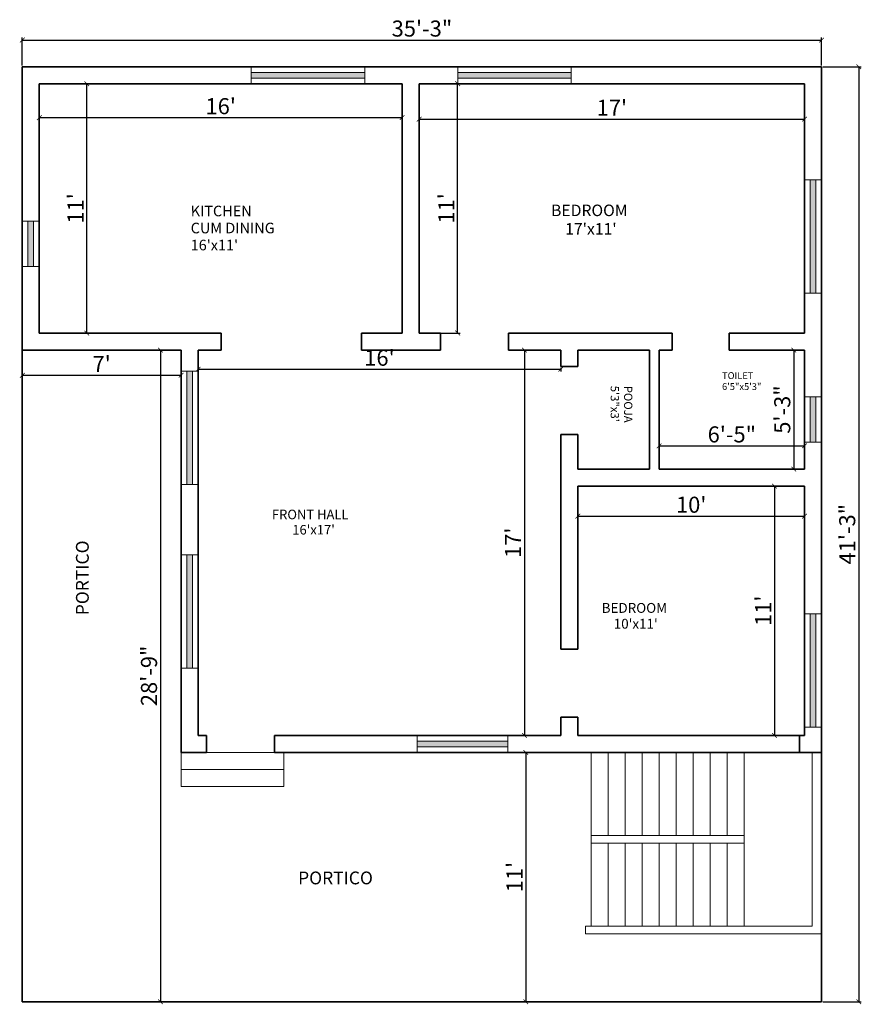
# Model space of a CAD drawing. Units: inches. Extents: x 3799 to 20199, y 1682 to 8087.
# Tile 14 of 30: x 7648 to 8094, y 5909 to 6430. Entities that reach past the tile are written whole.
import ezdxf

# ---------------------------------------------------------------- set-up
doc = ezdxf.new("R2010")
doc.units = ezdxf.units.IN
for name, color, linetype, lineweight in [('A-ANNO-DIMS', 2, 'Continuous', 18), ('A-AREA-IDEN', 7, 'Continuous', 18), ('A-FLOR-STRS', 41, 'Continuous', 18), ('A-GLAZ', 152, 'Continuous', 18), ('A-WALL', 7, 'Continuous', 35), ('A-WALL-PATT', 252, 'Continuous', 13)]:
    doc.layers.add(name, color=color, linetype=linetype, lineweight=lineweight)
doc.styles.get("Standard").update_dxf_attribs({"font": 'arial.ttf'})
doc.dimstyles.new('ISO-25', dxfattribs={"dimtxt": 8.5, "dimasz": 2.5, "dimexe": 1.25, "dimexo": 0.625, "dimtad": 1, "dimdec": 0, "dimlunit": 3, "dimtxsty": 'Standard', "dimblk": 'ARCHTICK', "dimcen": 2.5, "dimadec": 0, "dimazin": 0, "dimtfac": 1, "dimtdec": 0, "dimtmove": 0, "dimatfit": 3, "dimfxl": 1, "dimarcsym": 0})

# ---------------------------------------------------------------- blocks, each defined once
blk = doc.blocks.new('_ArchTick')
at = {"color": 0, "linetype": 'ByBlock', "const_width": 0.15}
blk.add_lwpolyline([(-0.5, -0.5), (0.5, 0.5)], dxfattribs=at)
blk = doc.blocks.new('*D200')
at = {"layer": 'A-ANNO-DIMS', "color": 0, "lineweight": -2, "transparency": 16777216}
for p, q in [((7658.6, 6395.56), (7658.6, 6376.97)), ((7850.6, 6395.56), (7850.6, 6376.97)), ((7658.6, 6378.22), (7850.6, 6378.22))]:
    blk.add_line(p, q, dxfattribs=at)
at = {"layer": 'Defpoints', "color": 0, "transparency": 16777216}
for p in [(7658.6, 6396.18), (7850.6, 6396.18), (7850.6, 6378.22)]:
    blk.add_point(p, dxfattribs=at)
at = {"layer": 'A-ANNO-DIMS', "color": 0, "lineweight": -2, "transparency": 16777216, "xscale": 2.5, "yscale": 2.5, "zscale": 2.5, "rotation": 180}
blk.add_blockref('_ArchTick', (7658.6, 6378.22), dxfattribs=at)
at = {"layer": 'A-ANNO-DIMS', "color": 0, "lineweight": -2, "transparency": 16777216, "xscale": 2.5, "yscale": 2.5, "zscale": 2.5}
blk.add_blockref('_ArchTick', (7850.6, 6378.22), dxfattribs=at)
at = {"layer": 'A-ANNO-DIMS', "color": 0, "transparency": 16777216, "insert": (7754.6, 6383.19), "char_height": 8.5, "attachment_point": 5}
blk.add_mtext("16'", dxfattribs=at)
blk = doc.blocks.new('*D201')
at = {"layer": 'A-ANNO-DIMS', "color": 0, "lineweight": -2, "transparency": 16777216}
for p, q in [((7659.22, 6396.18), (7685, 6396.18)), ((7683.75, 6264.18), (7683.75, 6396.18)), ((7659.22, 6264.18), (7685, 6264.18))]:
    blk.add_line(p, q, dxfattribs=at)
at = {"layer": 'Defpoints', "color": 0, "transparency": 16777216}
for p in [(7658.6, 6396.18), (7683.75, 6396.18), (7658.6, 6264.18)]:
    blk.add_point(p, dxfattribs=at)
at = {"layer": 'A-ANNO-DIMS', "color": 0, "lineweight": -2, "transparency": 16777216, "xscale": 2.5, "yscale": 2.5, "zscale": 2.5}
for p, rotation in [((7683.75, 6396.18), 90), ((7683.75, 6264.18), 270)]:
    blk.add_blockref('_ArchTick', p, dxfattribs=dict(at, rotation=rotation))
at = {"layer": 'A-ANNO-DIMS', "color": 0, "transparency": 16777216, "insert": (7678.86, 6330.18), "char_height": 8.5, "attachment_point": 5, "rotation": 90}
blk.add_mtext("11'", dxfattribs=at)
blk = doc.blocks.new('*D202')
at = {"layer": 'A-ANNO-DIMS', "color": 0, "lineweight": -2, "transparency": 16777216}
for p, q in [((7860.22, 6396.18), (7881.25, 6396.18)), ((7880, 6264.18), (7880, 6396.18)), ((7860.22, 6264.18), (7881.25, 6264.18))]:
    blk.add_line(p, q, dxfattribs=at)
at = {"layer": 'Defpoints', "color": 0, "transparency": 16777216}
for p in [(7859.6, 6396.18), (7880, 6396.18), (7859.6, 6264.18)]:
    blk.add_point(p, dxfattribs=at)
at = {"layer": 'A-ANNO-DIMS', "color": 0, "lineweight": -2, "transparency": 16777216, "xscale": 2.5, "yscale": 2.5, "zscale": 2.5}
for p, rotation in [((7880, 6396.18), 90), ((7880, 6264.18), 270)]:
    blk.add_blockref('_ArchTick', p, dxfattribs=dict(at, rotation=rotation))
at = {"layer": 'A-ANNO-DIMS', "color": 0, "transparency": 16777216, "insert": (7875.11, 6330.18), "char_height": 8.5, "attachment_point": 5, "rotation": 90}
blk.add_mtext("11'", dxfattribs=at)
blk = doc.blocks.new('*D203')
at = {"layer": 'A-ANNO-DIMS', "color": 0, "lineweight": -2, "transparency": 16777216}
for p, q in [((7859.6, 6395.56), (7859.6, 6376.2)), ((8063.6, 6395.56), (8063.6, 6376.2)), ((7859.6, 6377.45), (8063.6, 6377.45))]:
    blk.add_line(p, q, dxfattribs=at)
at = {"layer": 'Defpoints', "color": 0, "transparency": 16777216}
for p in [(7859.6, 6396.18), (8063.6, 6396.18), (8063.6, 6377.45)]:
    blk.add_point(p, dxfattribs=at)
at = {"layer": 'A-ANNO-DIMS', "color": 0, "lineweight": -2, "transparency": 16777216, "xscale": 2.5, "yscale": 2.5, "zscale": 2.5, "rotation": 180}
blk.add_blockref('_ArchTick', (7859.6, 6377.45), dxfattribs=at)
at = {"layer": 'A-ANNO-DIMS', "color": 0, "lineweight": -2, "transparency": 16777216, "xscale": 2.5, "yscale": 2.5, "zscale": 2.5}
blk.add_blockref('_ArchTick', (8063.6, 6377.45), dxfattribs=at)
at = {"layer": 'A-ANNO-DIMS', "color": 0, "transparency": 16777216, "insert": (7961.6, 6382.34), "char_height": 8.5, "attachment_point": 5}
blk.add_mtext("17'", dxfattribs=at)
blk = doc.blocks.new('*D204')
at = {"layer": 'A-ANNO-DIMS', "color": 0, "lineweight": -2, "transparency": 16777216}
for p, q in [((7986.6, 6192.81), (7986.6, 6205.71)), ((7986.6, 6204.46), (8063.6, 6204.46)), ((8063.6, 6192.81), (8063.6, 6205.71))]:
    blk.add_line(p, q, dxfattribs=at)
at = {"layer": 'Defpoints', "color": 0, "transparency": 16777216}
for p in [(8063.6, 6204.46), (7986.6, 6192.18), (8063.6, 6192.18)]:
    blk.add_point(p, dxfattribs=at)
at = {"layer": 'A-ANNO-DIMS', "color": 0, "lineweight": -2, "transparency": 16777216, "xscale": 2.5, "yscale": 2.5, "zscale": 2.5, "rotation": 180}
blk.add_blockref('_ArchTick', (7986.6, 6204.46), dxfattribs=at)
at = {"layer": 'A-ANNO-DIMS', "color": 0, "lineweight": -2, "transparency": 16777216, "xscale": 2.5, "yscale": 2.5, "zscale": 2.5}
blk.add_blockref('_ArchTick', (8063.6, 6204.46), dxfattribs=at)
at = {"layer": 'A-ANNO-DIMS', "color": 0, "transparency": 16777216, "insert": (8025.1, 6209.42), "char_height": 8.5, "attachment_point": 5}
blk.add_mtext('6\'-5"', dxfattribs=at)
blk = doc.blocks.new('*D205')
at = {"layer": 'A-ANNO-DIMS', "color": 0, "lineweight": -2, "transparency": 16777216}
for p, q in [((8062.97, 6255.18), (8056.61, 6255.18)), ((8057.86, 6255.18), (8057.86, 6192.18)), ((8062.97, 6192.18), (8056.61, 6192.18))]:
    blk.add_line(p, q, dxfattribs=at)
at = {"layer": 'Defpoints', "color": 0, "transparency": 16777216}
for p in [(8063.6, 6255.18), (8057.86, 6192.18), (8063.6, 6192.18)]:
    blk.add_point(p, dxfattribs=at)
at = {"layer": 'A-ANNO-DIMS', "color": 0, "lineweight": -2, "transparency": 16777216, "xscale": 2.5, "yscale": 2.5, "zscale": 2.5}
for p, rotation in [((8057.86, 6255.18), 90), ((8057.86, 6192.18), 270)]:
    blk.add_blockref('_ArchTick', p, dxfattribs=dict(at, rotation=rotation))
at = {"layer": 'A-ANNO-DIMS', "color": 0, "transparency": 16777216, "insert": (8052.9, 6223.68), "char_height": 8.5, "attachment_point": 5, "rotation": 90}
blk.add_mtext('5\'-3"', dxfattribs=at)
blk = doc.blocks.new('*D206')
at = {"layer": 'A-ANNO-DIMS', "color": 0, "lineweight": -2, "transparency": 16777216}
for p, q in [((7943.6, 6182.56), (7943.6, 6165.96)), ((8063.6, 6182.56), (8063.6, 6165.96)), ((7943.6, 6167.21), (8063.6, 6167.21))]:
    blk.add_line(p, q, dxfattribs=at)
at = {"layer": 'Defpoints', "color": 0, "transparency": 16777216}
for p in [(7943.6, 6183.18), (8063.6, 6183.18), (8063.6, 6167.21)]:
    blk.add_point(p, dxfattribs=at)
at = {"layer": 'A-ANNO-DIMS', "color": 0, "lineweight": -2, "transparency": 16777216, "xscale": 2.5, "yscale": 2.5, "zscale": 2.5, "rotation": 180}
blk.add_blockref('_ArchTick', (7943.6, 6167.21), dxfattribs=at)
at = {"layer": 'A-ANNO-DIMS', "color": 0, "lineweight": -2, "transparency": 16777216, "xscale": 2.5, "yscale": 2.5, "zscale": 2.5}
blk.add_blockref('_ArchTick', (8063.6, 6167.21), dxfattribs=at)
at = {"layer": 'A-ANNO-DIMS', "color": 0, "transparency": 16777216, "insert": (8003.6, 6172.18), "char_height": 8.5, "attachment_point": 5}
blk.add_mtext("10'", dxfattribs=at)
blk = doc.blocks.new('*D207')
at = {"layer": 'A-ANNO-DIMS', "color": 0, "lineweight": -2, "transparency": 16777216}
for p, q in [((8062.97, 6183.18), (8046.43, 6183.18)), ((8047.68, 6183.18), (8047.68, 6051.18)), ((8062.97, 6051.18), (8046.43, 6051.18))]:
    blk.add_line(p, q, dxfattribs=at)
at = {"layer": 'Defpoints', "color": 0, "transparency": 16777216}
for p in [(8063.6, 6183.18), (8047.68, 6051.18), (8063.6, 6051.18)]:
    blk.add_point(p, dxfattribs=at)
at = {"layer": 'A-ANNO-DIMS', "color": 0, "lineweight": -2, "transparency": 16777216, "xscale": 2.5, "yscale": 2.5, "zscale": 2.5}
for p, rotation in [((8047.68, 6183.18), 90), ((8047.68, 6051.18), 270)]:
    blk.add_blockref('_ArchTick', p, dxfattribs=dict(at, rotation=rotation))
at = {"layer": 'A-ANNO-DIMS', "color": 0, "transparency": 16777216, "insert": (8042.78, 6117.18), "char_height": 8.5, "attachment_point": 5, "rotation": 90}
blk.add_mtext("11'", dxfattribs=at)
blk = doc.blocks.new('*D208')
at = {"layer": 'A-ANNO-DIMS', "color": 0, "lineweight": -2, "transparency": 16777216}
for p, q in [((7742.6, 6244.54), (7742.6, 6246.29)), ((7742.6, 6245.04), (7934.6, 6245.04)), ((7934.6, 6245.81), (7934.6, 6243.79))]:
    blk.add_line(p, q, dxfattribs=at)
at = {"layer": 'Defpoints', "color": 0, "transparency": 16777216}
for p in [(7934.6, 6246.44), (7934.6, 6245.04), (7742.6, 6243.91)]:
    blk.add_point(p, dxfattribs=at)
at = {"layer": 'A-ANNO-DIMS', "color": 0, "lineweight": -2, "transparency": 16777216, "xscale": 2.5, "yscale": 2.5, "zscale": 2.5, "rotation": 180}
blk.add_blockref('_ArchTick', (7742.6, 6245.04), dxfattribs=at)
at = {"layer": 'A-ANNO-DIMS', "color": 0, "lineweight": -2, "transparency": 16777216, "xscale": 2.5, "yscale": 2.5, "zscale": 2.5}
blk.add_blockref('_ArchTick', (7934.6, 6245.04), dxfattribs=at)
at = {"layer": 'A-ANNO-DIMS', "color": 0, "transparency": 16777216, "insert": (7838.6, 6250.01), "char_height": 8.5, "attachment_point": 5}
blk.add_mtext("16'", dxfattribs=at)
blk = doc.blocks.new('*D209')
at = {"layer": 'A-ANNO-DIMS', "color": 0, "lineweight": -2, "transparency": 16777216}
for p, q in [((7907.56, 6255.18), (7916.55, 6255.18)), ((7915.3, 6255.18), (7915.3, 6051.18)), ((7907.17, 6051.18), (7916.55, 6051.18))]:
    blk.add_line(p, q, dxfattribs=at)
at = {"layer": 'Defpoints', "color": 0, "transparency": 16777216}
for p in [(7906.93, 6255.18), (7906.55, 6051.18), (7915.3, 6051.18)]:
    blk.add_point(p, dxfattribs=at)
at = {"layer": 'A-ANNO-DIMS', "color": 0, "lineweight": -2, "transparency": 16777216, "xscale": 2.5, "yscale": 2.5, "zscale": 2.5}
for p, rotation in [((7915.3, 6255.18), 90), ((7915.3, 6051.18), 270)]:
    blk.add_blockref('_ArchTick', p, dxfattribs=dict(at, rotation=rotation))
at = {"layer": 'A-ANNO-DIMS', "color": 0, "transparency": 16777216, "insert": (7910.41, 6153.18), "char_height": 8.5, "attachment_point": 5, "rotation": 90}
blk.add_mtext("17'", dxfattribs=at)
blk = doc.blocks.new('*D210')
at = {"layer": 'A-ANNO-DIMS', "color": 0, "lineweight": -2, "transparency": 16777216}
for p, q in [((7732.97, 6255.18), (7721.46, 6255.18)), ((7722.71, 6255.18), (7722.71, 5910.18)), ((7732.97, 5910.18), (7721.46, 5910.18))]:
    blk.add_line(p, q, dxfattribs=at)
at = {"layer": 'Defpoints', "color": 0, "transparency": 16777216}
for p in [(7733.6, 6255.18), (7722.71, 5910.18), (7733.6, 5910.18)]:
    blk.add_point(p, dxfattribs=at)
at = {"layer": 'A-ANNO-DIMS', "color": 0, "lineweight": -2, "transparency": 16777216, "xscale": 2.5, "yscale": 2.5, "zscale": 2.5}
for p, rotation in [((7722.71, 6255.18), 90), ((7722.71, 5910.18), 270)]:
    blk.add_blockref('_ArchTick', p, dxfattribs=dict(at, rotation=rotation))
at = {"layer": 'A-ANNO-DIMS', "color": 0, "transparency": 16777216, "insert": (7717.74, 6082.68), "char_height": 8.5, "attachment_point": 5, "rotation": 90}
blk.add_mtext('28\'-9"', dxfattribs=at)
blk = doc.blocks.new('*D211')
at = {"layer": 'A-ANNO-DIMS', "color": 0, "lineweight": -2, "transparency": 16777216}
for p, q in [((7649.6, 6254.56), (7649.6, 6240.56)), ((7733.6, 6254.56), (7733.6, 6240.56)), ((7649.6, 6241.81), (7733.6, 6241.81))]:
    blk.add_line(p, q, dxfattribs=at)
at = {"layer": 'Defpoints', "color": 0, "transparency": 16777216}
for p in [(7649.6, 6255.18), (7733.6, 6255.18), (7733.6, 6241.81)]:
    blk.add_point(p, dxfattribs=at)
at = {"layer": 'A-ANNO-DIMS', "color": 0, "lineweight": -2, "transparency": 16777216, "xscale": 2.5, "yscale": 2.5, "zscale": 2.5, "rotation": 180}
blk.add_blockref('_ArchTick', (7649.6, 6241.81), dxfattribs=at)
at = {"layer": 'A-ANNO-DIMS', "color": 0, "lineweight": -2, "transparency": 16777216, "xscale": 2.5, "yscale": 2.5, "zscale": 2.5}
blk.add_blockref('_ArchTick', (7733.6, 6241.81), dxfattribs=at)
at = {"layer": 'A-ANNO-DIMS', "color": 0, "transparency": 16777216, "insert": (7691.6, 6246.69), "char_height": 8.5, "attachment_point": 5}
blk.add_mtext("7'", dxfattribs=at)
blk = doc.blocks.new('*D212')
at = {"layer": 'A-ANNO-DIMS', "color": 0, "lineweight": -2, "transparency": 16777216}
for p, q in [((7907.17, 6042.18), (7917.32, 6042.18)), ((7916.07, 6042.18), (7916.07, 5910.18)), ((7907.17, 5910.18), (7917.32, 5910.18))]:
    blk.add_line(p, q, dxfattribs=at)
at = {"layer": 'Defpoints', "color": 0, "transparency": 16777216}
for p in [(7906.55, 6042.18), (7906.55, 5910.18), (7916.07, 5910.18)]:
    blk.add_point(p, dxfattribs=at)
at = {"layer": 'A-ANNO-DIMS', "color": 0, "lineweight": -2, "transparency": 16777216, "xscale": 2.5, "yscale": 2.5, "zscale": 2.5}
for p, rotation in [((7916.07, 6042.18), 90), ((7916.07, 5910.18), 270)]:
    blk.add_blockref('_ArchTick', p, dxfattribs=dict(at, rotation=rotation))
at = {"layer": 'A-ANNO-DIMS', "color": 0, "transparency": 16777216, "insert": (7911.18, 5976.18), "char_height": 8.5, "attachment_point": 5, "rotation": 90}
blk.add_mtext("11'", dxfattribs=at)
blk = doc.blocks.new('*D213')
at = {"layer": 'A-ANNO-DIMS', "color": 0, "lineweight": -2, "transparency": 16777216}
for p, q in [((8073.22, 6405.18), (8093.49, 6405.18)), ((8092.24, 6405.18), (8092.24, 5910.18)), ((8073.22, 5910.18), (8093.49, 5910.18))]:
    blk.add_line(p, q, dxfattribs=at)
at = {"layer": 'Defpoints', "color": 0, "transparency": 16777216}
for p in [(8072.6, 6405.18), (8072.6, 5910.18), (8092.24, 5910.18)]:
    blk.add_point(p, dxfattribs=at)
at = {"layer": 'A-ANNO-DIMS', "color": 0, "lineweight": -2, "transparency": 16777216, "xscale": 2.5, "yscale": 2.5, "zscale": 2.5}
for p, rotation in [((8092.24, 6405.18), 90), ((8092.24, 5910.18), 270)]:
    blk.add_blockref('_ArchTick', p, dxfattribs=dict(at, rotation=rotation))
at = {"layer": 'A-ANNO-DIMS', "color": 0, "transparency": 16777216, "insert": (8087.27, 6157.68), "char_height": 8.5, "attachment_point": 5, "rotation": 90}
blk.add_mtext('41\'-3"', dxfattribs=at)
blk = doc.blocks.new('*D214')
at = {"layer": 'A-ANNO-DIMS', "color": 0, "lineweight": -2, "transparency": 16777216}
for p, q in [((7649.6, 6405.81), (7649.6, 6420.57)), ((7649.6, 6419.32), (8072.6, 6419.32)), ((8072.6, 6405.81), (8072.6, 6420.57))]:
    blk.add_line(p, q, dxfattribs=at)
at = {"layer": 'Defpoints', "color": 0, "transparency": 16777216}
for p in [(8072.6, 6419.32), (7649.6, 6405.18), (8072.6, 6405.18)]:
    blk.add_point(p, dxfattribs=at)
at = {"layer": 'A-ANNO-DIMS', "color": 0, "lineweight": -2, "transparency": 16777216, "xscale": 2.5, "yscale": 2.5, "zscale": 2.5, "rotation": 180}
blk.add_blockref('_ArchTick', (7649.6, 6419.32), dxfattribs=at)
at = {"layer": 'A-ANNO-DIMS', "color": 0, "lineweight": -2, "transparency": 16777216, "xscale": 2.5, "yscale": 2.5, "zscale": 2.5}
blk.add_blockref('_ArchTick', (8072.6, 6419.32), dxfattribs=at)
at = {"layer": 'A-ANNO-DIMS', "color": 0, "transparency": 16777216, "insert": (7861.1, 6424.28), "char_height": 8.5, "attachment_point": 5}
blk.add_mtext('35\'-3"', dxfattribs=at)
blk = doc.blocks.new('WIN-24IN-9IN-FRAME')
for p, q in [((0, 24), (9, 24)), ((3, 0), (3, 24)), ((6, 0), (6, 24)), ((0, 0), (9, 0))]:
    blk.add_line(p, q)
blk = doc.blocks.new('WIN-48IN-9IN-FRAME')
for p, q in [((0, 0), (0, 9)), ((48, 6), (0, 6)), ((48, 0), (48, 9)), ((48, 3), (0, 3))]:
    blk.add_line(p, q)
blk = doc.blocks.new('WIN-60IN-9IN-FRAME')
for p, q in [((0, 9), (0, 0)), ((60, 6), (0, 6)), ((60, 9), (60, 0)), ((60, 3), (0, 3))]:
    blk.add_line(p, q)

msp = doc.modelspace()

# ---------------------------------------------------------------- hatches: boundary and pattern name
at = {"layer": 'A-WALL-PATT'}
h = msp.add_hatch(color=256, dxfattribs=at)
h.dxf.hatch_style = 1
h.paths.add_polyline_path([(7830.8, 6402.18), (7770.8, 6402.18), (7770.8, 6399.18), (7830.8, 6399.18)])
h.paths.add_polyline_path([(7940.06, 6402.18), (7880.06, 6402.18), (7880.06, 6399.18), (7940.06, 6399.18)])
h.paths.add_polyline_path([(8069.6, 6345.29), (8066.6, 6345.29), (8066.6, 6285.29), (8069.6, 6285.29)])
h.paths.add_polyline_path([(8069.6, 6230.39), (8066.6, 6230.39), (8066.6, 6206.39), (8069.6, 6206.39)])
h.paths.add_polyline_path([(8069.6, 6115.61), (8066.6, 6115.61), (8066.6, 6055.61), (8069.6, 6055.61)])
h.paths.add_polyline_path([(7906.55, 6048.18), (7858.55, 6048.18), (7858.55, 6045.18), (7906.55, 6045.18)])
h.paths.add_polyline_path([(7739.6, 6146.78), (7736.6, 6146.78), (7736.6, 6086.78), (7739.6, 6086.78)])
h.paths.add_polyline_path([(7739.6, 6243.91), (7736.6, 6243.91), (7736.6, 6183.91), (7739.6, 6183.91)])
h.paths.add_polyline_path([(7655.6, 6323.49), (7652.6, 6323.49), (7652.6, 6299.49), (7655.6, 6299.49)])

# ---------------------------------------------------------------- linework, layer by layer
at = {"layer": 'A-FLOR-STRS'}
for p, q in [((7733.6, 6042.18), (7783, 6042.18)), ((7733.6, 6042.18), (7733.6, 6024.18)), ((7788.04, 6042.18), (7788.04, 6024.18)), ((7950.69, 6042.18), (7950.69, 5950.18)), ((7959.69, 6042.18), (7959.69, 5998.18)), ((7968.69, 6042.18), (7968.69, 5998.18)), ((7977.69, 6042.18), (7977.69, 5998.18)), ((7986.69, 6042.18), (7986.69, 5998.18)), ((7995.69, 6042.18), (7995.69, 5998.18)), ((8004.69, 6042.18), (8004.69, 5998.18)), ((8013.69, 6042.18), (8013.69, 5998.18)), ((8022.69, 6042.18), (8022.69, 5998.18)), ((8031.69, 6042.18), (8031.69, 5950.18)), ((8067.6, 6042.18), (8067.6, 5950.18)), ((7733.6, 6033.18), (7788.04, 6033.18)), ((7733.6, 6024.18), (7788.04, 6024.18)), ((8031.69, 5998.18), (7950.69, 5998.18)), ((8031.69, 5994.18), (7950.69, 5994.18)), ((7959.69, 5994.18), (7959.69, 5950.18)), ((7968.69, 5994.18), (7968.69, 5950.18)), ((7977.69, 5994.18), (7977.69, 5950.18)), ((7986.69, 5994.18), (7986.69, 5950.18)), ((7995.69, 5994.18), (7995.69, 5950.18)), ((8004.69, 5994.18), (8004.69, 5950.18)), ((8013.69, 5994.18), (8013.69, 5950.18)), ((8022.69, 5994.18), (8022.69, 5950.18)), ((8067.6, 5950.18), (7947.69, 5950.18)), ((7947.69, 5950.18), (7947.69, 5946.18)), ((8072.6, 5946.18), (7947.69, 5946.18))]:
    msp.add_line(p, q, dxfattribs=at)
at = {"layer": 'A-WALL'}
for p, q in [((7649.6, 5910.18), (7649.6, 6405.18)), ((7649.6, 6405.18), (8072.6, 6405.18)), ((8072.6, 6405.18), (8072.6, 5910.18)), ((7658.6, 6396.18), (7850.6, 6396.18)), ((7658.6, 6264.18), (7658.6, 6396.18)), ((7850.6, 6264.18), (7850.6, 6396.18)), ((7859.6, 6264.18), (7859.6, 6396.18)), ((7859.6, 6396.18), (8063.6, 6396.18)), ((8063.6, 6396.18), (8063.6, 6264.18)), ((7658.6, 6264.18), (7754.81, 6264.18)), ((7754.81, 6255.18), (7754.81, 6264.18)), ((7829.04, 6264.18), (7829.04, 6255.18)), ((7829.04, 6264.18), (7850.6, 6264.18)), ((7859.6, 6264.18), (7870.93, 6264.18)), ((7870.93, 6264.18), (7870.93, 6255.18)), ((7906.93, 6264.18), (7906.93, 6255.18)), ((7906.93, 6264.18), (7993.61, 6264.18)), ((7993.61, 6255.18), (7993.61, 6264.18)), ((8023.61, 6255.18), (8023.61, 6264.18)), ((8023.61, 6264.18), (8063.6, 6264.18)), ((7649.6, 6255.18), (7733.6, 6255.18)), ((7733.6, 6042.18), (7733.6, 6255.18)), ((7742.6, 6255.18), (7754.81, 6255.18)), ((7742.6, 6051.18), (7742.6, 6255.18)), ((7829.04, 6255.18), (7870.93, 6255.18)), ((7906.93, 6255.18), (7934.6, 6255.18)), ((7934.6, 6246.44), (7934.6, 6255.18)), ((7943.6, 6255.18), (7981.6, 6255.18)), ((7943.6, 6246.44), (7943.6, 6255.18)), ((7981.6, 6255.18), (7981.6, 6192.18)), ((7986.6, 6255.18), (7986.6, 6192.18)), ((7986.6, 6255.18), (7993.61, 6255.18)), ((8023.61, 6255.18), (8063.6, 6255.18)), ((8063.6, 6255.18), (8063.6, 6192.18)), ((7943.6, 6246.44), (7934.6, 6246.44)), ((7943.6, 6210.44), (7934.6, 6210.44)), ((7934.6, 6096.84), (7934.6, 6210.44)), ((7943.6, 6192.18), (7943.6, 6210.44)), ((7943.6, 6192.18), (7981.6, 6192.18)), ((7986.6, 6192.18), (8063.6, 6192.18)), ((7943.6, 6183.18), (8063.6, 6183.18)), ((7943.6, 6096.84), (7943.6, 6183.18)), ((8063.6, 6183.18), (8063.6, 6051.18)), ((7943.6, 6096.84), (7934.6, 6096.84)), ((7934.6, 6051.18), (7934.6, 6060.84)), ((7943.6, 6060.84), (7934.6, 6060.84)), ((7943.6, 6051.18), (7943.6, 6060.84)), ((7742.6, 6051.18), (7747, 6051.18)), ((7747, 6051.18), (7747, 6042.18)), ((7783, 6051.18), (7783, 6042.18)), ((7783, 6051.18), (7934.6, 6051.18)), ((7943.6, 6051.18), (8063.6, 6051.18)), ((8060.95, 6051.18), (8060.95, 6042.18)), ((7733.6, 6042.18), (7747, 6042.18)), ((7783, 6042.18), (8072.6, 6042.18)), ((8072.6, 5910.18), (7649.6, 5910.18))]:
    msp.add_line(p, q, dxfattribs=at)

# ---------------------------------------------------------------- block references
at = {"layer": 'A-GLAZ'}
for name, p in [('WIN-60IN-9IN-FRAME', (7770.8, 6396.18)), ('WIN-60IN-9IN-FRAME', (7880.06, 6396.18)), ('WIN-24IN-9IN-FRAME', (7649.6, 6299.49)), ('WIN-24IN-9IN-FRAME', (8063.6, 6206.39)), ('WIN-48IN-9IN-FRAME', (7858.55, 6042.18))]:
    msp.add_blockref(name, p, dxfattribs=at)
at = {"layer": 'A-GLAZ', "rotation": 90}
for p in [(8072.6, 6285.29), (7742.6, 6183.91), (7742.6, 6086.78), (8072.6, 6055.61)]:
    msp.add_blockref('WIN-60IN-9IN-FRAME', p, dxfattribs=at)

# ---------------------------------------------------------------- texts
at = {"layer": 'A-AREA-IDEN'}
for s, height, rotation, p in [('KITCHEN', 5.612, 0.0167, (7738.72, 6325.98)), ('BEDROOM', 6.101, 0.0167, (7929.43, 6326.07)), ('CUM DINING', 5.612, 0.0167, (7738.72, 6316.97)), ("    17'x11'", 6.1013, 0.0167, (7929.43, 6316.27)), ("16'x11'", 5.612, 0.0167, (7738.72, 6307.95)), ('TOILET', 3.617, 0.0167, (8019.92, 6239.84)), ('5\'3"x3\'', 4.398, 270.0167, (7960.98, 6236.29)), ('POOJA', 4.398, 270.0167, (7968.05, 6236.29)), ('6\'5"x5\'3"', 3.617, 0.0167, (8019.92, 6234.03)), ('FRONT HALL', 5.038, 0.0167, (7781.71, 6165.61)), ("       16'x17'", 5.0379, 0.0167, (7781.71, 6157.52)), ('PORTICO', 6.778, 90.0167, (7684.77, 6114.79)), ('BEDROOM', 5.21, 0.0167, (7956.24, 6116.04)), ("    10'x11'", 5.2104, 0.0167, (7956.25, 6107.67)), ('PORTICO', 6.778, 0.0167, (7795.55, 5972.31))]:
    msp.add_text(s, height=height, rotation=rotation, dxfattribs=at).set_placement(p)

# ---------------------------------------------------------------- dimensions: what is measured, and where the dimension line sits
at = {"layer": 'A-ANNO-DIMS'}
for base, p1, p2, picture, middle in [((8072.6, 6419.32), (7649.6, 6405.18), (8072.6, 6405.18), '*D214', (7861.1, 6424.28)), ((7850.6, 6378.22), (7658.6, 6396.18), (7850.6, 6396.18), '*D200', (7754.6, 6383.19)), ((8063.6, 6377.45), (7859.6, 6396.18), (8063.6, 6396.18), '*D203', (7961.6, 6382.34)), ((7934.6, 6245.04), (7742.6, 6243.91), (7934.6, 6246.44), '*D208', (7838.6, 6250.01)), ((7733.6, 6241.81), (7649.6, 6255.18), (7733.6, 6255.18), '*D211', (7691.6, 6246.69)), ((8063.6, 6204.46), (7986.6, 6192.18), (8063.6, 6192.18), '*D204', (8025.1, 6209.42)), ((8063.6, 6167.21), (7943.6, 6183.18), (8063.6, 6183.18), '*D206', (8003.6, 6172.18))]:
    dim = msp.add_linear_dim(base=base, p1=p1, p2=p2, dimstyle='ISO-25', override={"dimclrd": 0, "dimclre": 0, "dimclrt": 0}, dxfattribs=at)
    dim.commit()
    dim.dimension.update_dxf_attribs({"geometry": picture, "text_midpoint": middle})
for base, p1, p2, picture, middle in [((8092.24, 5910.18), (8072.6, 6405.18), (8072.6, 5910.18), '*D213', (8087.27, 6157.68)), ((7683.75, 6396.18), (7658.6, 6264.18), (7658.6, 6396.18), '*D201', (7678.86, 6330.18)), ((7880, 6396.18), (7859.6, 6264.18), (7859.6, 6396.18), '*D202', (7875.11, 6330.18)), ((7722.71, 5910.18), (7733.6, 6255.18), (7733.6, 5910.18), '*D210', (7717.74, 6082.68)), ((7915.3, 6051.18), (7906.93, 6255.18), (7906.55, 6051.18), '*D209', (7910.41, 6153.18)), ((8057.86, 6192.18), (8063.6, 6255.18), (8063.6, 6192.18), '*D205', (8052.9, 6223.68)), ((8047.68, 6051.18), (8063.6, 6183.18), (8063.6, 6051.18), '*D207', (8042.78, 6117.18)), ((7916.07, 5910.18), (7906.55, 6042.18), (7906.55, 5910.18), '*D212', (7911.18, 5976.18))]:
    dim = msp.add_linear_dim(base=base, p1=p1, p2=p2, angle=90, dimstyle='ISO-25', override={"dimclrd": 0, "dimclre": 0, "dimclrt": 0}, dxfattribs=at)
    dim.commit()
    dim.dimension.update_dxf_attribs({"geometry": picture, "text_midpoint": middle})

doc.saveas('drawing.dxf')
